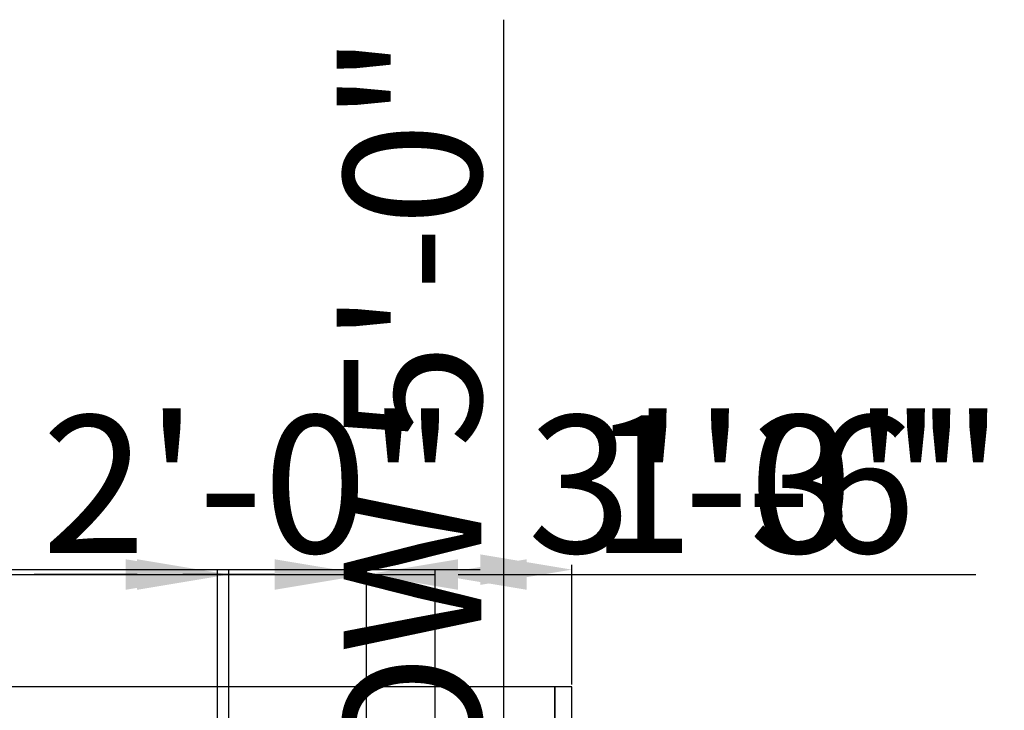
# Model space of a CAD drawing. Units: inches. Extents: x 1041 to 1781, y -140 to 732.
# Tile 6 of 6: x 1359 to 1616, y 506 to 687. Entities that reach past the tile are written whole.
import ezdxf

# ---------------------------------------------------------------- set-up
doc = ezdxf.new("R2010")
doc.units = ezdxf.units.IN
for name, color, linetype, lineweight in [('A-WALL', 7, 'Continuous', 35), ('C-PROP', 3, 'Continuous', 25), ('dimension', 130, 'Continuous', 18)]:
    doc.layers.add(name, color=color, linetype=linetype, lineweight=lineweight)
doc.styles.get("Standard").update_dxf_attribs({"font": 'arial.ttf'})
doc.dimstyles.new('ISO-25', dxfattribs={"dimtxt": 36, "dimasz": 24, "dimexe": 1.25, "dimexo": 0.625, "dimtad": 1, "dimlunit": 4, "dimtxsty": 'Standard', "dimcen": 2.5, "dimadec": 0, "dimazin": 0, "dimtfac": 1, "dimtmove": 0, "dimatfit": 3, "dimfxl": 1, "dimarcsym": 0})

# ---------------------------------------------------------------- blocks, each defined once
blk = doc.blocks.new('*D1')
at = {"layer": 'Defpoints', "color": 0, "transparency": 16777216}
for p in [(1503.25, 542.96), (1143.25, 512.23), (1503.25, 512.23)]:
    blk.add_point(p, dxfattribs=at)
at = {"layer": 'dimension', "color": 0, "lineweight": -2, "transparency": 16777216}
for p, q in [((1143.25, 512.86), (1143.25, 544.21)), ((1503.25, 512.86), (1503.25, 544.21)), ((1167.25, 542.96), (1479.25, 542.96))]:
    blk.add_line(p, q, dxfattribs=at)
at = {"layer": 'dimension', "color": 0, "transparency": 16777216}
for points in [[(1167.25, 546.96), (1167.25, 538.96), (1143.25, 542.96)], [(1479.25, 546.96), (1479.25, 538.96), (1503.25, 542.96)]]:
    blk.add_solid(points, dxfattribs=at)
at = {"layer": 'dimension', "color": 0, "transparency": 16777216, "insert": (1323.25, 561.98), "char_height": 36, "attachment_point": 5}
blk.add_mtext("30'", dxfattribs=at)
blk = doc.blocks.new('*D13')
at = {"layer": 'Defpoints', "color": 0, "transparency": 16777216}
for p in [(1476.44, 329.99), (1485.44, 329.99), (1476.44, 269.99)]:
    blk.add_point(p, dxfattribs=at)
at = {"layer": 'dimension', "color": 0, "lineweight": -2, "transparency": 16777216}
for p, q in [((1485.44, 329.99), (1485.44, 687.05)), ((1477.06, 329.99), (1486.69, 329.99)), ((1485.44, 293.99), (1485.44, 305.99)), ((1477.06, 269.99), (1486.69, 269.99))]:
    blk.add_line(p, q, dxfattribs=at)
at = {"layer": 'dimension', "color": 0, "transparency": 16777216}
for points in [[(1481.44, 305.99), (1489.44, 305.99), (1485.44, 329.99)], [(1481.44, 293.99), (1489.44, 293.99), (1485.44, 269.99)]]:
    blk.add_solid(points, dxfattribs=at)
at = {"layer": 'dimension', "color": 0, "transparency": 16777216, "insert": (1466.19, 520.52), "char_height": 36, "attachment_point": 5, "rotation": 90}
blk.add_mtext('WINDOW 5\'-0"', dxfattribs=at)
blk = doc.blocks.new('*D18')
at = {"layer": 'Defpoints', "color": 0, "transparency": 16777216}
for p in [(1449.44, 541.68), (1413.44, 207.73), (1449.44, 207.73)]:
    blk.add_point(p, dxfattribs=at)
at = {"layer": 'dimension', "color": 0, "lineweight": -2, "transparency": 16777216}
for p, q in [((1389.44, 541.68), (1365.44, 541.68)), ((1413.44, 208.36), (1413.44, 542.93)), ((1413.44, 541.68), (1449.44, 541.68)), ((1449.44, 208.36), (1449.44, 542.93)), ((1473.44, 541.68), (1594.36, 541.68))]:
    blk.add_line(p, q, dxfattribs=at)
at = {"layer": 'dimension', "color": 0, "transparency": 16777216}
for points in [[(1389.44, 545.68), (1389.44, 537.68), (1413.44, 541.68)], [(1473.44, 545.68), (1473.44, 537.68), (1449.44, 541.68)]]:
    blk.add_solid(points, dxfattribs=at)
at = {"layer": 'dimension', "color": 0, "transparency": 16777216, "insert": (1545.9, 560.7), "char_height": 36, "attachment_point": 5}
blk.add_mtext('3\'-0"', dxfattribs=at)
blk = doc.blocks.new('*D21')
at = {"layer": 'Defpoints', "color": 0, "transparency": 16777216}
for p in [(1449.44, 541.68), (1410.44, 41.23), (1449.44, 41.23)]:
    blk.add_point(p, dxfattribs=at)
at = {"layer": 'dimension', "color": 0, "lineweight": -2, "transparency": 16777216}
for p, q in [((1386.44, 541.68), (1362.44, 541.68)), ((1410.44, 41.86), (1410.44, 542.93)), ((1410.44, 541.68), (1449.44, 541.68)), ((1449.44, 41.86), (1449.44, 542.93)), ((1473.44, 541.68), (1594.36, 541.68))]:
    blk.add_line(p, q, dxfattribs=at)
at = {"layer": 'dimension', "color": 0, "transparency": 16777216}
for points in [[(1386.44, 545.68), (1386.44, 537.68), (1410.44, 541.68)], [(1473.44, 545.68), (1473.44, 537.68), (1449.44, 541.68)]]:
    blk.add_solid(points, dxfattribs=at)
at = {"layer": 'dimension', "color": 0, "transparency": 16777216, "insert": (1545.9, 560.7), "char_height": 36, "attachment_point": 5}
blk.add_mtext('3\'-3"', dxfattribs=at)
blk = doc.blocks.new('*D35')
at = {"layer": 'Defpoints', "color": 0, "transparency": 16777216}
for p in [(1321.94, 541.68), (1297.94, 165.73), (1321.94, 165.73)]:
    blk.add_point(p, dxfattribs=at)
at = {"layer": 'dimension', "color": 0, "lineweight": -2, "transparency": 16777216}
for p, q in [((1273.94, 541.68), (1249.94, 541.68)), ((1297.94, 166.36), (1297.94, 542.93)), ((1297.94, 541.68), (1321.94, 541.68)), ((1321.94, 166.36), (1321.94, 542.93)), ((1345.94, 541.68), (1467.5, 541.68))]:
    blk.add_line(p, q, dxfattribs=at)
at = {"layer": 'dimension', "color": 0, "transparency": 16777216}
for points in [[(1273.94, 545.68), (1273.94, 537.68), (1297.94, 541.68)], [(1345.94, 545.68), (1345.94, 537.68), (1321.94, 541.68)]]:
    blk.add_solid(points, dxfattribs=at)
at = {"layer": 'dimension', "color": 0, "transparency": 16777216, "insert": (1418.72, 560.69), "char_height": 36, "attachment_point": 5}
blk.add_mtext('2\'-0"', dxfattribs=at)
blk = doc.blocks.new('*D39')
at = {"layer": 'Defpoints', "color": 0, "transparency": 16777216}
for p in [(1467.44, 541.68), (1449.44, 207.73), (1467.44, 207.73)]:
    blk.add_point(p, dxfattribs=at)
at = {"layer": 'dimension', "color": 0, "lineweight": -2, "transparency": 16777216}
for p, q in [((1425.44, 541.68), (1401.44, 541.68)), ((1449.44, 208.36), (1449.44, 542.93)), ((1449.44, 541.68), (1467.44, 541.68)), ((1467.44, 208.36), (1467.44, 542.93)), ((1491.44, 541.68), (1609, 541.68))]:
    blk.add_line(p, q, dxfattribs=at)
at = {"layer": 'dimension', "color": 0, "transparency": 16777216}
for points in [[(1425.44, 545.68), (1425.44, 537.68), (1449.44, 541.68)], [(1491.44, 545.68), (1491.44, 537.68), (1467.44, 541.68)]]:
    blk.add_solid(points, dxfattribs=at)
at = {"layer": 'dimension', "color": 0, "transparency": 16777216, "insert": (1562.22, 560.69), "char_height": 36, "attachment_point": 5}
blk.add_mtext('1\'-6"', dxfattribs=at)

msp = doc.modelspace()

# ---------------------------------------------------------------- linework, layer by layer
at = {"layer": 'A-WALL'}
msp.add_line((1498.749, 32.233), (1498.749, 512.233), dxfattribs=at)
at = {"layer": 'C-PROP'}
for p, q in [((1503.249, 512.233), (1143.249, 512.233)), ((1503.249, 32.233), (1503.249, 512.233))]:
    msp.add_line(p, q, dxfattribs=at)

# ---------------------------------------------------------------- dimensions: what is measured, and where the dimension line sits
at = {"layer": 'dimension'}
dim = msp.add_linear_dim(base=(1485.438, 329.99), p1=(1476.438, 269.99), p2=(1476.438, 329.99), angle=90, text='WINDOW <>', dimstyle='ISO-25', override={"dimdec": 1, "dimlfac": 1, "dimrnd": 0, "dimzin": 1, "dimdsep": 46, "dimlunit": 4, "dimfrac": 2}, dxfattribs=at)
dim.commit()
dim.dimension.update_dxf_attribs({"geometry": '*D13', "text_midpoint": (1466.186, 520.519)})
for base, p1, p2, override, picture, middle in [((1503.249, 542.957), (1143.249, 512.233), (1503.249, 512.233), {"dimclrd": 0, "dimclre": 0, "dimclrt": 0}, '*D1', (1323.249, 561.975)), ((1321.938, 541.683), (1297.938, 165.733), (1321.938, 165.733), {"dimdec": 1, "dimlfac": 1, "dimrnd": 0, "dimzin": 1, "dimdsep": 46, "dimlunit": 4, "dimfrac": 2}, '*D35', (1418.718, 560.688)), ((1449.438, 541.683), (1410.438, 41.233), (1449.438, 41.233), {"dimdec": 1, "dimlfac": 1, "dimrnd": 0, "dimzin": 1, "dimdsep": 46, "dimlunit": 4, "dimfrac": 2}, '*D21', (1545.899, 560.7)), ((1449.438, 541.683), (1413.438, 207.733), (1449.438, 207.733), {"dimdec": 1, "dimlfac": 1, "dimrnd": 0, "dimzin": 1, "dimdsep": 46, "dimlunit": 4, "dimfrac": 2}, '*D18', (1545.899, 560.7)), ((1467.438, 541.683), (1449.438, 207.733), (1467.438, 207.733), {"dimdec": 1, "dimlfac": 1, "dimrnd": 0, "dimzin": 1, "dimdsep": 46, "dimlunit": 4, "dimfrac": 2}, '*D39', (1562.217, 560.688))]:
    dim = msp.add_linear_dim(base=base, p1=p1, p2=p2, dimstyle='ISO-25', override=override, dxfattribs=at)
    dim.commit()
    dim.dimension.update_dxf_attribs({"geometry": picture, "text_midpoint": middle})

doc.saveas('drawing.dxf')
